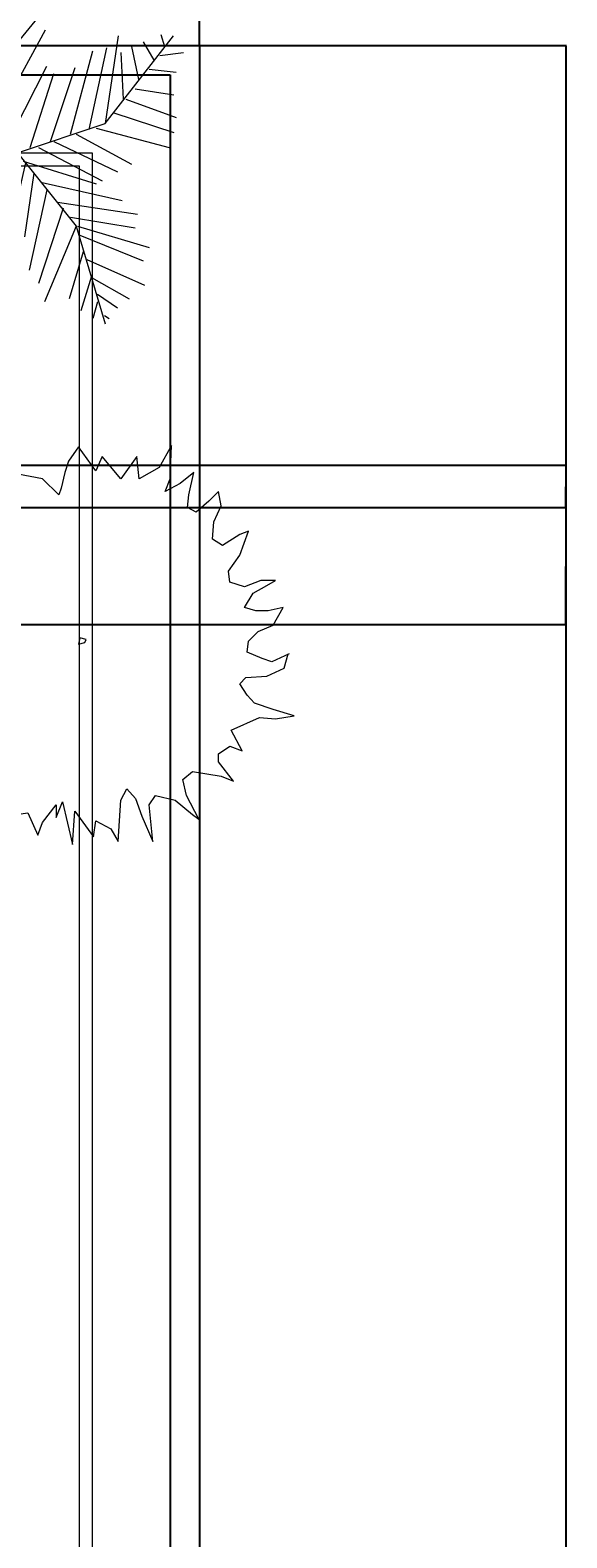
# Model space of a CAD drawing. Units: inches. Extents: x -4843 to -3402, y -164 to 3629.
# Tile 21 of 22: x -3994 to -3829, y 691 to 1154. Entities that reach past the tile are written whole.
import ezdxf

# ---------------------------------------------------------------- set-up
doc = ezdxf.new("R2010")
doc.units = ezdxf.units.IN
for name, color, linetype, lineweight in [('A-ANNO-DIMS', 2, 'Continuous', 18), ('C-PROP', 7, 'Continuous', 25), ('L-PLNT-EDGE', 7, 'Continuous', 18), ('PLANTS', 3, 'Continuous', 13)]:
    doc.layers.add(name, color=color, linetype=linetype, lineweight=lineweight)
doc.styles.get("Standard").update_dxf_attribs({"font": 'arial.ttf'})
doc.dimstyles.get("Standard").update_dxf_attribs({"dimtxt": 0.18, "dimasz": 0.18, "dimexe": 0.18, "dimexo": 0.0625, "dimgap": 0.09, "dimtad": 0, "dimtih": 1, "dimtoh": 1, "dimdec": 4, "dimzin": 0, "dimdsep": 46, "dimtxsty": 'Standard', "dimcen": 0.09, "dimadec": 0, "dimazin": 0, "dimtfac": 1, "dimtdec": 4, "dimtofl": 0, "dimtmove": 0, "dimatfit": 3, "dimfxl": 1, "dimtolj": 1, "dimtzin": 0, "dimarcsym": 0})

# ---------------------------------------------------------------- blocks, each defined once
blk = doc.blocks.new('*U33')
for p, q in [((-258.7244, 1362.456), (-332.3336, 1421.4348)), ((0, 0), (-266.7, 1447.8)), ((-231.1146, 1315.2628), (-166.7002, 1421.4348)), ((-221.9198, 1197.3052), (-433.5526, 1338.8594)), ((-185.1152, 1008.5578), (-553.1612, 1185.4942)), ((-194.31, 1102.9442), (-65.4812, 1256.284)), ((-148.3106, 914.1968), (118.5418, 1220.9018)), ((-129.8956, 701.8528), (265.7602, 1185.4942)), ((-129.8956, 713.6638), (-626.7704, 1032.1544)), ((-74.7014, 418.7444), (219.7608, 961.39)), ((-93.091, 489.5342), (-700.3796, 902.3858)), ((685.8, 228.6), (1219.2, 914.4)), ((689.0258, 230.0224), (790.2448, 914.1968)), ((891.4384, 831.6214), (946.658, 572.1096)), ((983.4626, 867.0036), (1066.2666, 725.4494)), ((1121.4862, 925.9824), (1149.0706, 831.6214)), ((-1234.059, 536.7274), (-1252.4486, 737.2604)), ((-1105.2302, 725.4494), (-1077.6458, 395.1732)), ((-902.8176, 713.6638), (-617.5756, 100.2538)), ((412.9786, 147.447), (587.8068, 796.2392)), ((560.197, 182.8292), (698.2206, 819.8358)), ((808.6344, 784.4282), (827.0494, 418.7444)), ((1112.2914, 760.8316), (1296.3144, 784.4282)), ((-800.1, 114.3), (-1333.5, 647.7)), ((-976.4268, 666.4706), (-884.4026, 194.6402)), ((-369.1382, 53.086), (-783.1836, 642.874)), ((-617.5756, 607.4918), (-74.7014, 347.98)), ((-28.6766, 171.0436), (228.9556, 678.2816)), ((100.1268, 41.275), (284.1498, 619.2774)), ((256.5654, 88.4682), (449.7832, 666.4706)), ((1029.462, 654.685), (1241.0948, 631.0884)), ((-1206.4492, 501.3198), (-1418.082, 465.9376)), ((919.0482, 501.3198), (1222.6798, 454.152)), ((845.439, 418.7444), (1241.0948, 277.1902)), ((-1031.621, 347.98), (-1399.667, 277.1902)), ((-525.5514, 347.98), (-28.6766, 123.8504)), ((753.4148, 312.5978), (1222.6798, 159.2326)), ((-847.598, 159.2326), (-1326.0578, 135.636)), ((0, 0), (685.8, 228.6)), ((458.978, 147.447), (891.4384, -88.4682)), ((615.4166, 194.6402), (1185.8752, 41.275)), ((-718.7946, 88.4682), (-1215.644, -147.447)), ((-543.9664, 76.6572), (-967.2066, -206.4512)), ((0, 0), (-800.1, 114.3)), ((-405.9428, 53.086), (-764.794, -241.8334)), ((0, 0), (-571.5, -495.3)), ((-166.7002, 29.4894), (-543.9664, -206.4512)), ((0, 0), (457.2, -571.5)), ((164.5412, 41.275), (661.416, -218.2368)), ((284.1498, 88.4682), (781.0246, -147.447)), ((-120.7008, -88.4682), (-93.091, -371.5766)), ((63.3222, -76.6826), (-37.8714, -513.1308)), ((44.9326, -64.897), (615.4166, -241.8334)), ((-166.7002, -147.447), (-507.1618, -253.619)), ((-240.3094, -218.2368), (-157.5054, -595.7062)), ((127.7366, -159.258), (54.1274, -654.685)), ((192.151, -230.0224), (817.8292, -371.5766)), ((-387.5278, -324.4088), (-764.794, -324.4088)), ((-341.5284, -289.0012), (-221.9198, -831.6214)), ((228.9556, -289.0012), (90.932, -914.1968)), ((-442.7474, -383.3876), (-1086.8406, -477.7486)), ((-525.5514, -465.963), (-451.9422, -1126.5408)), ((-433.5526, -383.3876), (-323.1134, -1020.3688)), ((357.759, -430.5554), (164.5412, -1020.3688)), ((311.7596, -383.3876), (937.4378, -477.7486)), ((-617.5756, -548.5384), (-1077.6458, -560.324)), ((-571.5, -495.3), (-952.5, -1143)), ((458.978, -572.1096), (210.5406, -1161.923)), ((412.9786, -501.3452), (919.0482, -583.9206)), ((457.2, -571.5), (685.8, -1333.5)), ((468.1982, -572.1096), (1029.462, -737.2604)), ((-681.9646, -666.496), (-1022.4262, -654.685)), ((-635.9652, -607.5172), (-580.771, -1150.1374)), ((486.5878, -642.8994), (983.4626, -843.4324)), ((-718.7946, -737.2604), (-1086.8406, -796.2392)), ((-737.1842, -784.4536), (-709.5744, -1114.7298)), ((514.1976, -772.6426), (403.7838, -1138.3264)), ((-783.1836, -867.029), (-1077.6458, -902.4112)), ((-829.2084, -937.7934), (-810.7934, -1126.5408)), ((541.8074, -831.6214), (992.6574, -1032.1544)), ((-875.2078, -1008.5832), (-1040.8412, -1079.3476)), ((578.612, -961.39), (495.7826, -1232.7128)), ((578.612, -973.1756), (873.0488, -1138.3264)), ((624.6114, -1161.923), (587.8068, -1291.6916)), ((624.6114, -1102.9442), (781.0246, -1209.1162)), ((679.8056, -1268.095), (716.6102, -1291.6916))]:
    blk.add_line(p, q)
blk = doc.blocks.new('*U34')
for points in [[(0, 1540.256), (-77.4954, 1428.4452), (-106.5784, 1341.501), (-135.636, 1217.295), (-155.0162, 1167.6126), (-280.9748, 1291.8186), (-474.7514, 1329.0804), (-532.892, 1204.8744), (-513.5118, 1105.5096), (-523.1892, 1006.1194), (-658.8506, 1093.089), (-707.2884, 1254.5568), (-842.9244, 1329.0804), (-775.1064, 1204.8744), (-794.4866, 1093.089), (-765.429, 968.8576), (-852.6272, 894.334), (-1036.701, 931.5958), (-1249.8832, 968.8576), (-1191.7426, 931.5958), (-1075.4614, 807.3898), (-1075.4614, 720.4456), (-1182.0398, 695.6044), (-1414.5768, 695.6044), (-1269.238, 558.9524), (-1385.5192, 534.1112), (-1172.3624, 372.6434), (-1307.9984, 285.6992), (-1521.1552, 285.6992), (-1414.5768, 223.5962), (-1366.139, 136.652), (-1453.3372, 86.9442), (-1540.5354, -37.2618), (-1550.2382, -124.206), (-1501.775, -86.9442), (-1385.5192, -37.2618), (-1307.9984, -111.7854), (-1346.7588, -260.8326), (-1501.775, -385.064), (-1249.8832, -335.3816), (-1482.3948, -621.0554), (-1230.503, -534.1112), (-1104.5444, -571.373), (-1094.8416, -658.3172), (-1201.42, -794.9692), (-1094.8416, -770.128), (-1230.503, -1006.1194), (-978.5858, -807.3898), (-1036.701, -919.1752), (-823.5442, -944.0164), (-852.6272, -1105.4842), (-901.065, -1254.5568), (-726.6686, -1142.746), (-600.71, -1180.0078), (-561.9496, -1316.6598), (-552.2722, -1465.707), (-484.4542, -1329.0804), (-397.2306, -1316.6598), (-319.7352, -1490.5482), (-280.9748, -1391.1834), (-174.3964, -1254.5568), (-174.3964, -1353.9216), (-125.9586, -1229.7156), (-48.4378, -1565.0718), (-29.0576, -1304.2392), (116.2812, -1502.9688), (135.6614, -1378.7628), (251.9172, -1440.8658), (310.0578, -1540.2306), (329.438, -1217.295), (377.8758, -1130.3254), (445.6938, -1204.8744), (494.157, -1341.501), (581.3552, -1540.2306), (552.2722, -1254.5568), (600.71, -1180.0078), (755.7516, -1217.295), (891.3876, -1329.0804), (939.8254, -1366.3422), (842.9498, -1180.0078), (813.8668, -1055.8018), (891.3876, -993.6988), (1114.2472, -1030.9606), (1211.1228, -1068.2224), (1094.867, -919.1752), (1094.867, -857.0722), (1182.0652, -794.9692), (1278.9408, -832.231), (1191.7426, -670.7378), (1414.6022, -571.373), (1540.5608, -583.7936), (1685.8996, -558.9524), (1521.1806, -509.27), (1375.8418, -459.5876), (1317.7012, -397.4846), (1259.5606, -310.515), (1308.0238, -260.8326), (1472.7174, -248.412), (1608.3788, -186.309), (1637.4364, -74.5236)], [(1647.1392, -74.5236), (1511.4778, -136.6266), (1433.9824, -111.7854), (1317.7012, -62.103), (1327.404, 24.8412), (1404.8994, 99.3648), (1521.1806, 149.0726), (1598.676, 285.6992), (1482.4202, 260.858), (1385.5192, 260.858), (1298.321, 285.6992), (1366.139, 397.4846), (1472.7174, 459.5876), (1540.5608, 496.8494), (1424.2796, 496.8494), (1298.321, 447.167), (1182.0652, 484.4288), (1172.3624, 571.3984), (1259.5606, 695.6044), (1327.404, 881.9134), (1259.5606, 857.0722), (1123.9246, 770.128), (1046.4038, 819.8104), (1056.1066, 956.437), (1114.2472, 1080.6684), (1094.867, 1192.4538), (1017.3462, 1117.9302), (920.4452, 1030.9606), (852.6272, 1068.2478), (862.33, 1167.6126), (901.0904, 1341.501), (794.512, 1254.5568), (678.2308, 1192.4538), (716.9912, 1291.8186), (726.6686, 1552.6766), (629.793, 1378.7628), (474.7768, 1291.8186), (455.3966, 1465.7324), (329.438, 1291.8186), (184.0992, 1465.7324), (135.6614, 1353.9216), (0, 1540.256)]]:
    blk.add_lwpolyline(points)
blk.add_lwpolyline([(9.7028, 49.6824), (0, 0), (48.4378, 12.4206), (58.1406, 37.2618)], close=True)
blk = doc.blocks.new('*D60')
at = {"layer": 'A-ANNO-DIMS', "color": 0, "lineweight": -2, "transparency": 16777216}
for p, q in [((-4723.78, 1149.42), (-4723.78, 1392.95)), ((-4723.6, 1392.77), (-4333.07, 1392.77)), ((-3941.96, 1392.77), (-4332.5, 1392.77)), ((-3941.78, 1149.42), (-3941.78, 1392.95))]:
    blk.add_line(p, q, dxfattribs=at)
at = {"layer": 'A-ANNO-DIMS', "color": 0, "transparency": 16777216}
for points in [[(-4723.6, 1392.8), (-4723.6, 1392.74), (-4723.78, 1392.77)], [(-3941.96, 1392.8), (-3941.96, 1392.74), (-3941.78, 1392.77)]]:
    blk.add_solid(points, dxfattribs=at)
at = {"layer": 'Defpoints', "color": 0, "transparency": 16777216}
for p in [(-3941.78, 1392.77), (-4723.78, 1149.35), (-3941.78, 1149.35)]:
    blk.add_point(p, dxfattribs=at)
at = {"layer": 'A-ANNO-DIMS', "color": 0, "transparency": 16777216, "insert": (-4332.78, 1392.77), "char_height": 0.18, "attachment_point": 5}
blk.add_mtext('\\A1;782', dxfattribs=at)
blk = doc.blocks.new('*D61')
at = {"layer": 'A-ANNO-DIMS', "color": 0, "lineweight": -2, "transparency": 16777216}
for p, q in [((-3941.72, 1149.35), (-3828.78, 1149.35)), ((-3828.96, 1149.17), (-3828.96, 618.04)), ((-3828.96, 86.53), (-3828.96, 617.67)), ((-3941.72, 86.35), (-3828.78, 86.35))]:
    blk.add_line(p, q, dxfattribs=at)
at = {"layer": 'A-ANNO-DIMS', "color": 0, "transparency": 16777216}
for points in [[(-3828.99, 1149.17), (-3828.93, 1149.17), (-3828.96, 1149.35)], [(-3828.99, 86.53), (-3828.93, 86.53), (-3828.96, 86.35)]]:
    blk.add_solid(points, dxfattribs=at)
at = {"layer": 'Defpoints', "color": 0, "transparency": 16777216}
for p in [(-3941.78, 1149.35), (-3828.96, 1149.35), (-3941.78, 86.35)]:
    blk.add_point(p, dxfattribs=at)
at = {"layer": 'A-ANNO-DIMS', "color": 0, "transparency": 16777216, "insert": (-3828.96, 617.85), "char_height": 0.18, "attachment_point": 5}
blk.add_mtext('\\A1;1063', dxfattribs=at)
blk = doc.blocks.new('*D77')
at = {"layer": 'A-ANNO-DIMS', "color": 0, "lineweight": -2, "transparency": 16777216}
for p, q in [((-4181.72, 1020.35), (-3828.78, 1020.35)), ((-3828.96, 1020.17), (-3828.96, 1014.04)), ((-3828.96, 1007.53), (-3828.96, 1013.67)), ((-4181.72, 1007.35), (-3828.78, 1007.35))]:
    blk.add_line(p, q, dxfattribs=at)
at = {"layer": 'A-ANNO-DIMS', "color": 0, "transparency": 16777216}
for points in [[(-3828.99, 1020.17), (-3828.93, 1020.17), (-3828.96, 1020.35)], [(-3828.99, 1007.53), (-3828.93, 1007.53), (-3828.96, 1007.35)]]:
    blk.add_solid(points, dxfattribs=at)
at = {"layer": 'Defpoints', "color": 0, "transparency": 16777216}
for p in [(-4181.78, 1020.35), (-4181.78, 1007.35), (-3828.96, 1007.35)]:
    blk.add_point(p, dxfattribs=at)
at = {"layer": 'A-ANNO-DIMS', "color": 0, "transparency": 16777216, "insert": (-3828.96, 1013.85), "char_height": 0.18, "attachment_point": 5}
blk.add_mtext('\\A1;13', dxfattribs=at)
blk = doc.blocks.new('*D78')
at = {"layer": 'A-ANNO-DIMS', "color": 0, "lineweight": -2, "transparency": 16777216}
for p, q in [((-4181.72, 1007.35), (-3828.78, 1007.35)), ((-3828.96, 1007.17), (-3828.96, 989.54)), ((-3828.96, 971.53), (-3828.96, 989.17)), ((-4181.72, 971.35), (-3828.78, 971.35))]:
    blk.add_line(p, q, dxfattribs=at)
at = {"layer": 'A-ANNO-DIMS', "color": 0, "transparency": 16777216}
for points in [[(-3828.99, 1007.17), (-3828.93, 1007.17), (-3828.96, 1007.35)], [(-3828.99, 971.53), (-3828.93, 971.53), (-3828.96, 971.35)]]:
    blk.add_solid(points, dxfattribs=at)
at = {"layer": 'Defpoints', "color": 0, "transparency": 16777216}
for p in [(-4181.78, 1007.35), (-4181.78, 971.35), (-3828.96, 971.35)]:
    blk.add_point(p, dxfattribs=at)
at = {"layer": 'A-ANNO-DIMS', "color": 0, "transparency": 16777216, "insert": (-3828.96, 989.35), "char_height": 0.18, "attachment_point": 5}
blk.add_mtext('\\A1;36', dxfattribs=at)

msp = doc.modelspace()

# ---------------------------------------------------------------- linework, layer by layer
at = {"layer": 'C-PROP'}
for p, q in [((-4723.78, 1149.35), (-3941.78, 1149.35)), ((-3941.78, 1149.35), (-3941.78, 86.35)), ((-4714.78, 1140.35), (-3950.78, 1140.35)), ((-3950.78, 1140.35), (-3950.78, 95.35))]:
    msp.add_line(p, q, dxfattribs=at)
at = {"layer": 'L-PLNT-EDGE'}
for p, q in [((-4696.78, 1116.35), (-3974.78, 1116.35)), ((-3974.78, 1116.35), (-3974.78, 95.35)), ((-4696.78, 1112.35), (-3978.78, 1112.35)), ((-3978.78, 1112.35), (-3978.78, 95.35))]:
    msp.add_line(p, q, dxfattribs=at)

# ---------------------------------------------------------------- block references
at = {"layer": 'PLANTS', "xscale": 0.0393700787401575, "yscale": 0.0393700787401575, "zscale": 0.0393700787401575}
for name, p in [('*U33', (-3997.76, 1116.35)), ('*U34', (-3978.97, 965.32))]:
    msp.add_blockref(name, p, dxfattribs=at)

# ---------------------------------------------------------------- dimensions: what is measured, and where the dimension line sits
at = {"layer": 'A-ANNO-DIMS'}
dim = msp.add_linear_dim(base=(-3941.78, 1392.77), p1=(-4723.78, 1149.35), p2=(-3941.78, 1149.35), dimstyle='Standard', override={"dimdec": 0, "dimlfac": 1, "dimrnd": 0, "dimzin": 0, "dimdsep": 46, "dimlunit": 2}, dxfattribs=at)
dim.commit()
dim.dimension.update_dxf_attribs({"geometry": '*D60', "text_midpoint": (-4332.78, 1392.77)})
for base, p1, p2, picture, middle in [((-3828.96, 1149.35), (-3941.78, 86.35), (-3941.78, 1149.35), '*D61', (-3828.96, 617.85)), ((-3828.96, 1007.35), (-4181.78, 1020.35), (-4181.78, 1007.35), '*D77', (-3828.96, 1013.85)), ((-3828.96, 971.35), (-4181.78, 1007.35), (-4181.78, 971.35), '*D78', (-3828.96, 989.35))]:
    dim = msp.add_linear_dim(base=base, p1=p1, p2=p2, angle=90, dimstyle='Standard', override={"dimdec": 0, "dimlfac": 1, "dimrnd": 0, "dimzin": 0, "dimdsep": 46, "dimlunit": 2}, dxfattribs=at)
    dim.commit()
    dim.dimension.update_dxf_attribs({"geometry": picture, "text_midpoint": middle})

doc.saveas('drawing.dxf')
